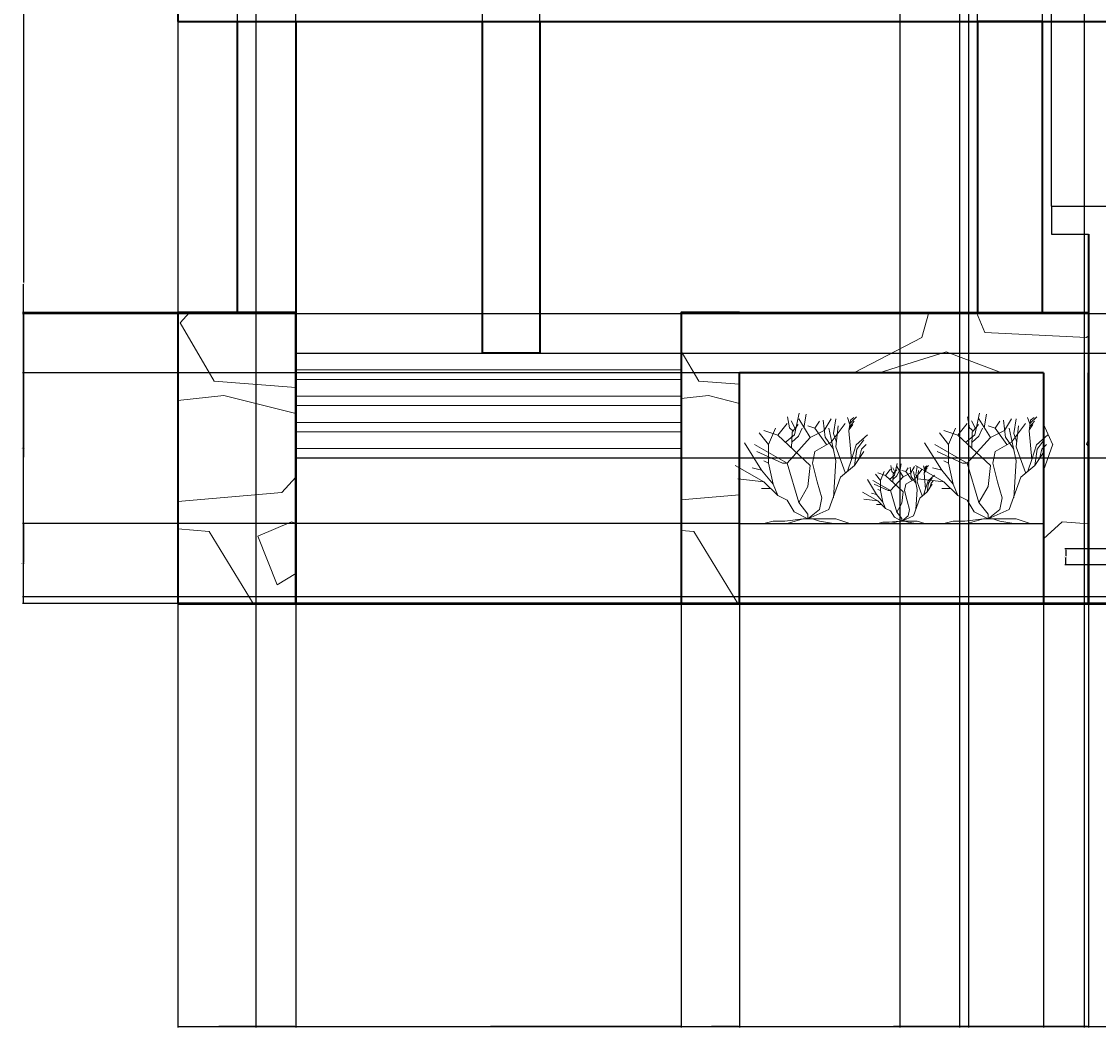
# Model space of a CAD drawing. Units: inches. Extents: x -8 to 554, y -200 to 499.
# Tile 1 of 12: x -8 to 214, y -200 to 7. Entities that reach past the tile are written whole.
import ezdxf

# ---------------------------------------------------------------- set-up
doc = ezdxf.new("R2010")
doc.units = ezdxf.units.IN
doc.header["$MEASUREMENT"] = 0
for name, color, linetype, lineweight in [('A-ANNO-DIMS', 2, 'Continuous', 18), ('A-COLS', 1, 'Continuous', 35), ('A-DOOR-GATE', 3, 'Continuous', 25), ('A-FLOR', 7, 'Continuous', 35), ('A-WALL', 7, 'Continuous', 35), ('A-WALL-PATT', 252, 'Continuous', 13), ('A-WALL-PRPT', 7, 'Continuous', 25), ('A-WALL-SCRN', 8, 'Continuous', 18), ('C-TOPO', 7, 'Continuous', 50), ('L-PLNT-TREE', 94, 'Continuous', 13)]:
    doc.layers.add(name, color=color, linetype=linetype, lineweight=lineweight)
doc.styles.get("Standard").update_dxf_attribs({"font": 'arial.ttf'})
doc.dimstyles.get("Standard").update_dxf_attribs({"dimtxt": 0.18, "dimasz": 0.18, "dimexe": 0.18, "dimexo": 0.0625, "dimgap": 0.09, "dimtad": 0, "dimtih": 1, "dimtoh": 1, "dimdec": 4, "dimzin": 0, "dimdsep": 46, "dimtxsty": 'Standard', "dimcen": 0.09, "dimadec": 0, "dimazin": 0, "dimtfac": 1, "dimtdec": 4, "dimtofl": 0, "dimtmove": 0, "dimatfit": 3, "dimfxl": 1, "dimtolj": 1, "dimtzin": 0, "dimarcsym": 0})

# ---------------------------------------------------------------- blocks, each defined once
blk = doc.blocks.new('*U2')
for p, q in [((-11.433, 18.289), (-10.457, 22.749)), ((-9.48, 19.775), (-8.992, 22.592)), ((-14.88, 18.24), (-12.96, 20.64)), ((-12.471, 19.775), (-12.898, 22.044)), ((-11.28, 19.619), (-12.104, 21.184)), ((-11.921, 18.836), (-10.64, 20.401)), ((-8.16, 17.76), (-10.56, 21.6)), ((-7.2, 19.68), (-8.64, 20.16)), ((-7.2, 19.68), (-6.24, 21.12)), ((-5.086, 17.741), (-5.513, 21.34)), ((-5.28, 19.2), (-3.84, 21.6)), ((-3.84, 16.8), (-0.96, 20.64)), ((-3.377, 18.602), (-2.888, 21.575)), ((-2.88, 15.84), (-2.4, 20.16)), ((-0.508, 21.888), (-0.081, 20.558)), ((-0.203, 19.149), (0.102, 21.34)), ((-0.142, 19.384), (0.59, 20.401)), ((-0.02, 20.01), (0.896, 21.105)), ((0.041, 20.714), (1.384, 22.044)), ((0.102, 21.34), (0.835, 21.888)), ((-16.8, 16.32), (-18.72, 18.72)), ((-14.88, 18.24), (-17.76, 19.2)), ((-16.8, 16.32), (-15.36, 19.68)), ((-8.16, 12), (-14.88, 18.24)), ((-13.325, 16.724), (-11.433, 18.289)), ((-11.677, 19.071), (-12.471, 19.775)), ((-12.043, 15.628), (-11.921, 18.836)), ((-11.982, 16.802), (-10.579, 18.054)), ((-10.579, 18.054), (-9.846, 19.697)), ((-8.16, 17.76), (-5.28, 19.2)), ((-4.8, 16.32), (-7.2, 19.68)), ((-3.377, 15.315), (-5.086, 17.819)), ((-2.88, 12.96), (-4.32, 19.68)), ((-2.766, 16.802), (-3.377, 18.602)), ((0.346, 13.203), (-0.203, 19.149)), ((1.323, 16.254), (3.642, 18.289)), ((-18.24, 11.04), (-21.755, 16.655)), ((-12.96, 12.48), (-19.68, 16.32)), ((-16.8, 12.48), (-16.8, 16.32)), ((-12.96, 12.48), (-8.16, 17.76)), ((-7.2, 14.88), (-3.84, 16.8)), ((-0.96, 10.56), (-2.88, 15.84)), ((0.346, 13.203), (1.323, 16.254)), ((1.44, 15.36), (2.88, 17.28)), ((2.4, 15.36), (3.36, 16.32)), ((-13.92, 12.48), (-19.2, 14.88)), ((-7.68, 12.48), (-7.2, 14.88)), ((0.96, 12), (1.44, 15.36)), ((0.96, 12), (2.88, 14.88)), ((1.92, 13.44), (2.4, 15.36)), ((-17.76, 8.64), (-23.663, 11.961)), ((-18.24, 11.04), (-20.16, 11.52)), ((-16.8, 12.48), (-17.76, 12.96)), ((-15.84, 8.16), (-16.8, 12.48)), ((-12.96, 12.48), (-13.92, 12.48)), ((-10.56, 4.32), (-12.96, 12.48)), ((-8.64, 7.68), (-8.16, 12)), ((-6.72, 8.64), (-7.68, 12.48)), ((-3.36, 5.28), (-2.88, 12.96)), ((-1.92, 9.6), (0.96, 12)), ((-0.48, 10.8), (0.346, 13.203)), ((-17.76, 8.64), (-23.128, 9.222)), ((-15.84, 8.16), (-18.24, 11.04)), ((-4.32, 2.88), (-1.92, 9.6)), ((-16.32, 7.2), (-18.24, 7.2)), ((-14.88, 5.76), (-17.76, 8.64)), ((-14.88, 5.76), (-15.84, 8.16)), ((-10.56, 4.32), (-8.64, 7.68)), ((-5.76, 5.28), (-6.72, 8.64)), ((-12.96, 4.8), (-14.88, 5.76)), ((-11.52, 2.4), (-12.96, 4.8)), ((-6.24, 2.88), (-5.76, 5.28)), ((-8.64, 0.96), (-11.52, 2.4)), ((-8.64, 1.92), (-10.56, 4.32)), ((-8.64, 0.96), (-4.32, 2.88)), ((-8.64, 0.96), (-6.24, 2.88)), ((-15.84, 0.48), (-17.76, 0)), ((-13.44, 0.48), (-15.84, 0.48)), ((-9.6, 0.96), (-13.44, 0.48)), ((-9.6, 0.96), (-12.96, 0)), ((-9.6, 0.96), (-7.68, 0.96)), ((-8.64, 0.96), (-8.64, 1.92)), ((-8.64, 0.96), (-2.88, 0.96)), ((-7.68, 0.96), (-6.24, 0.48)), ((-6.24, 0.48), (-3.36, 0)), ((-2.88, 0.96), (0, 0))]:
    blk.add_line(p, q)
blk = doc.blocks.new('GATE-PIER-ELEV')
blk.add_lwpolyline([(0, 76.14), (0, 0), (11.66, 0), (11.66, 76.14)])
blk = doc.blocks.new('*D15')
at = {"layer": 'A-ANNO-DIMS', "color": 0, "lineweight": -2, "transparency": 16777216}
for p, q in [((228.57, -101.26), (207.36, -101.26)), ((207.54, -101.44), (207.54, -102.71)), ((207.54, -104.35), (207.54, -103.08)), ((228.57, -104.53), (207.36, -104.53))]:
    blk.add_line(p, q, dxfattribs=at)
at = {"layer": 'A-ANNO-DIMS', "color": 0, "transparency": 16777216}
for points in [[(207.51, -101.44), (207.57, -101.44), (207.54, -101.26)], [(207.51, -104.35), (207.57, -104.35), (207.54, -104.53)]]:
    blk.add_solid(points, dxfattribs=at)
at = {"layer": 'Defpoints', "color": 0, "transparency": 16777216}
for p in [(207.54, -101.26), (228.63, -101.26), (228.63, -104.53)]:
    blk.add_point(p, dxfattribs=at)
at = {"layer": 'A-ANNO-DIMS', "color": 0, "transparency": 16777216, "insert": (207.54, -102.9), "char_height": 0.18, "attachment_point": 5}
blk.add_mtext('\\A1;3 TYP.', dxfattribs=at)
blk = doc.blocks.new('*D31')
at = {"layer": 'A-ANNO-DIMS', "color": 0, "lineweight": -2, "transparency": 16777216}
for p, q in [((24.34, 127.42), (24.34, -199.97)), ((453.32, -30.73), (453.32, -199.97)), ((24.52, -199.79), (238.54, -199.79)), ((453.14, -199.79), (239.12, -199.79))]:
    blk.add_line(p, q, dxfattribs=at)
at = {"layer": 'A-ANNO-DIMS', "color": 0, "transparency": 16777216}
for points in [[(24.52, -199.76), (24.52, -199.82), (24.34, -199.79)], [(453.14, -199.76), (453.14, -199.82), (453.32, -199.79)]]:
    blk.add_solid(points, dxfattribs=at)
at = {"layer": 'Defpoints', "color": 0, "transparency": 16777216}
for p in [(24.34, 127.48), (453.32, -30.67), (453.32, -199.79)]:
    blk.add_point(p, dxfattribs=at)
at = {"layer": 'A-ANNO-DIMS', "color": 0, "transparency": 16777216, "insert": (238.83, -199.79), "char_height": 0.18, "attachment_point": 5}
blk.add_mtext('\\A1;429', dxfattribs=at)
blk = doc.blocks.new('*D32')
at = {"layer": 'A-ANNO-DIMS', "color": 0, "lineweight": -2, "transparency": 16777216}
for p, q in [((24.34, 223.42), (24.34, -199.97)), ((444.34, 223.42), (444.34, -199.97)), ((24.52, -199.79), (234.05, -199.79)), ((444.16, -199.79), (234.63, -199.79))]:
    blk.add_line(p, q, dxfattribs=at)
at = {"layer": 'A-ANNO-DIMS', "color": 0, "transparency": 16777216}
for points in [[(24.52, -199.76), (24.52, -199.82), (24.34, -199.79)], [(444.16, -199.76), (444.16, -199.82), (444.34, -199.79)]]:
    blk.add_solid(points, dxfattribs=at)
at = {"layer": 'Defpoints', "color": 0, "transparency": 16777216}
for p in [(24.34, 223.48), (444.34, 223.48), (444.34, -199.79)]:
    blk.add_point(p, dxfattribs=at)
at = {"layer": 'A-ANNO-DIMS', "color": 0, "transparency": 16777216, "insert": (234.34, -199.79), "char_height": 0.18, "attachment_point": 5}
blk.add_mtext('\\A1;420', dxfattribs=at)
blk = doc.blocks.new('*D33')
at = {"layer": 'A-ANNO-DIMS', "color": 0, "lineweight": -2, "transparency": 16777216}
for p, q in [((36.28, 19.48), (-7.69, 19.48)), ((-7.51, 19.3), (-7.51, -46.34)), ((-7.51, -112.34), (-7.51, -46.7)), ((24.28, -112.52), (-7.69, -112.52))]:
    blk.add_line(p, q, dxfattribs=at)
at = {"layer": 'A-ANNO-DIMS', "color": 0, "transparency": 16777216}
for points in [[(-7.54, 19.3), (-7.48, 19.3), (-7.51, 19.48)], [(-7.54, -112.34), (-7.48, -112.34), (-7.51, -112.52)]]:
    blk.add_solid(points, dxfattribs=at)
at = {"layer": 'Defpoints', "color": 0, "transparency": 16777216}
for p in [(-7.51, 19.48), (36.34, 19.48), (24.34, -112.52)]:
    blk.add_point(p, dxfattribs=at)
at = {"layer": 'A-ANNO-DIMS', "color": 0, "transparency": 16777216, "insert": (-7.51, -46.52), "char_height": 0.18, "attachment_point": 5}
blk.add_mtext('\\A1;132', dxfattribs=at)
blk = doc.blocks.new('*D41')
at = {"layer": 'A-ANNO-DIMS', "color": 0, "lineweight": -2, "transparency": 16777216}
for p, q in [((24.34, 235.42), (24.34, -199.97)), ((40.45, 235.42), (40.45, -199.97)), ((24.52, -199.79), (31.94, -199.79)), ((40.27, -199.79), (32.85, -199.79))]:
    blk.add_line(p, q, dxfattribs=at)
at = {"layer": 'A-ANNO-DIMS', "color": 0, "transparency": 16777216}
for points in [[(24.52, -199.76), (24.52, -199.82), (24.34, -199.79)], [(40.27, -199.76), (40.27, -199.82), (40.45, -199.79)]]:
    blk.add_solid(points, dxfattribs=at)
at = {"layer": 'Defpoints', "color": 0, "transparency": 16777216}
for p in [(24.34, 235.48), (40.45, 235.48), (40.45, -199.79)]:
    blk.add_point(p, dxfattribs=at)
at = {"layer": 'A-ANNO-DIMS', "color": 0, "transparency": 16777216, "insert": (32.4, -199.79), "char_height": 0.18, "attachment_point": 5}
blk.add_mtext('\\A1;16.113', dxfattribs=at)
blk = doc.blocks.new('*D48')
at = {"layer": 'A-ANNO-DIMS', "color": 0, "lineweight": -2, "transparency": 16777216}
for p, q in [((24.34, -112.58), (24.34, -199.97)), ((48.69, -112.58), (48.69, -199.97)), ((24.52, -199.79), (36.05, -199.79)), ((48.51, -199.79), (36.98, -199.79))]:
    blk.add_line(p, q, dxfattribs=at)
at = {"layer": 'A-ANNO-DIMS', "color": 0, "transparency": 16777216}
for points in [[(24.52, -199.76), (24.52, -199.82), (24.34, -199.79)], [(48.51, -199.76), (48.51, -199.82), (48.69, -199.79)]]:
    blk.add_solid(points, dxfattribs=at)
at = {"layer": 'Defpoints', "color": 0, "transparency": 16777216}
for p in [(24.34, -112.52), (48.69, -112.52), (48.69, -199.79)]:
    blk.add_point(p, dxfattribs=at)
at = {"layer": 'A-ANNO-DIMS', "color": 0, "transparency": 16777216, "insert": (36.52, -199.79), "char_height": 0.18, "attachment_point": 5}
blk.add_mtext('\\A1;24.346', dxfattribs=at)
blk = doc.blocks.new('*D49')
at = {"layer": 'A-ANNO-DIMS', "color": 0, "lineweight": -2, "transparency": 16777216}
for p, q in [((48.69, -112.58), (48.69, -199.97)), ((128.23, -112.58), (128.23, -199.97)), ((48.87, -199.79), (88.07, -199.79)), ((128.05, -199.79), (88.85, -199.79))]:
    blk.add_line(p, q, dxfattribs=at)
at = {"layer": 'A-ANNO-DIMS', "color": 0, "transparency": 16777216}
for points in [[(48.87, -199.76), (48.87, -199.82), (48.69, -199.79)], [(128.05, -199.76), (128.05, -199.82), (128.23, -199.79)]]:
    blk.add_solid(points, dxfattribs=at)
at = {"layer": 'Defpoints', "color": 0, "transparency": 16777216}
for p in [(48.69, -112.52), (128.23, -112.52), (128.23, -199.79)]:
    blk.add_point(p, dxfattribs=at)
at = {"layer": 'A-ANNO-DIMS', "color": 0, "transparency": 16777216, "insert": (88.46, -199.79), "char_height": 0.18, "attachment_point": 5}
blk.add_mtext('\\A1;79.54', dxfattribs=at)
blk = doc.blocks.new('*D50')
at = {"layer": 'A-ANNO-DIMS', "color": 0, "lineweight": -2, "transparency": 16777216}
for p, q in [((128.23, -112.58), (128.23, -199.97)), ((140.23, -112.58), (140.23, -199.97)), ((128.41, -199.79), (134.02, -199.79)), ((140.05, -199.79), (134.44, -199.79))]:
    blk.add_line(p, q, dxfattribs=at)
at = {"layer": 'A-ANNO-DIMS', "color": 0, "transparency": 16777216}
for points in [[(128.41, -199.76), (128.41, -199.82), (128.23, -199.79)], [(140.05, -199.76), (140.05, -199.82), (140.23, -199.79)]]:
    blk.add_solid(points, dxfattribs=at)
at = {"layer": 'Defpoints', "color": 0, "transparency": 16777216}
for p in [(128.23, -112.52), (140.23, -112.52), (140.23, -199.79)]:
    blk.add_point(p, dxfattribs=at)
at = {"layer": 'A-ANNO-DIMS', "color": 0, "transparency": 16777216, "insert": (134.23, -199.79), "char_height": 0.18, "attachment_point": 5}
blk.add_mtext('\\A1;12', dxfattribs=at)
blk = doc.blocks.new('*D51')
at = {"layer": 'A-ANNO-DIMS', "color": 0, "lineweight": -2, "transparency": 16777216}
for p, q in [((140.23, -112.58), (140.23, -199.97)), ((202.92, -112.58), (202.92, -199.97)), ((140.41, -199.79), (171.18, -199.79)), ((202.74, -199.79), (171.97, -199.79))]:
    blk.add_line(p, q, dxfattribs=at)
at = {"layer": 'A-ANNO-DIMS', "color": 0, "transparency": 16777216}
for points in [[(140.41, -199.76), (140.41, -199.82), (140.23, -199.79)], [(202.74, -199.76), (202.74, -199.82), (202.92, -199.79)]]:
    blk.add_solid(points, dxfattribs=at)
at = {"layer": 'Defpoints', "color": 0, "transparency": 16777216}
for p in [(140.23, -112.52), (202.92, -112.52), (202.92, -199.79)]:
    blk.add_point(p, dxfattribs=at)
at = {"layer": 'A-ANNO-DIMS', "color": 0, "transparency": 16777216, "insert": (171.57, -199.79), "char_height": 0.18, "attachment_point": 5}
blk.add_mtext('\\A1;62.69', dxfattribs=at)
blk = doc.blocks.new('*D52')
at = {"layer": 'A-ANNO-DIMS', "color": 0, "lineweight": -2, "transparency": 16777216}
for p, q in [((202.92, -112.58), (202.92, -199.97)), ((212.23, -112.58), (212.23, -199.97)), ((203.1, -199.79), (207.18, -199.79)), ((212.05, -199.79), (207.97, -199.79))]:
    blk.add_line(p, q, dxfattribs=at)
at = {"layer": 'A-ANNO-DIMS', "color": 0, "transparency": 16777216}
for points in [[(203.1, -199.76), (203.1, -199.82), (202.92, -199.79)], [(212.05, -199.76), (212.05, -199.82), (212.23, -199.79)]]:
    blk.add_solid(points, dxfattribs=at)
at = {"layer": 'Defpoints', "color": 0, "transparency": 16777216}
for p in [(202.92, -112.52), (212.23, -112.52), (212.23, -199.79)]:
    blk.add_point(p, dxfattribs=at)
at = {"layer": 'A-ANNO-DIMS', "color": 0, "transparency": 16777216, "insert": (207.57, -199.79), "char_height": 0.18, "attachment_point": 5}
blk.add_mtext('\\A1;9.307', dxfattribs=at)
blk = doc.blocks.new('*D54')
at = {"layer": 'A-ANNO-DIMS', "color": 0, "lineweight": -2, "transparency": 16777216}
for p, q in [((24.28, -52.52), (-7.69, -52.52)), ((-7.51, -52.7), (-7.51, -82.34)), ((-7.51, -112.34), (-7.51, -82.7)), ((24.28, -112.52), (-7.69, -112.52))]:
    blk.add_line(p, q, dxfattribs=at)
at = {"layer": 'A-ANNO-DIMS', "color": 0, "transparency": 16777216}
for points in [[(-7.54, -52.7), (-7.48, -52.7), (-7.51, -52.52)], [(-7.54, -112.34), (-7.48, -112.34), (-7.51, -112.52)]]:
    blk.add_solid(points, dxfattribs=at)
at = {"layer": 'Defpoints', "color": 0, "transparency": 16777216}
for p in [(-7.51, -52.52), (24.34, -52.52), (24.34, -112.52)]:
    blk.add_point(p, dxfattribs=at)
at = {"layer": 'A-ANNO-DIMS', "color": 0, "transparency": 16777216, "insert": (-7.51, -82.52), "char_height": 0.18, "attachment_point": 5}
blk.add_mtext('\\A1;60', dxfattribs=at)
blk = doc.blocks.new('*D55')
at = {"layer": 'A-ANNO-DIMS', "color": 0, "lineweight": -2, "transparency": 16777216}
for p, q in [((204.61, -30.61), (204.61, 498.99)), ((204.79, 498.81), (328.57, 498.81)), ((453.14, 498.81), (329.36, 498.81)), ((453.32, -30.61), (453.32, 498.99))]:
    blk.add_line(p, q, dxfattribs=at)
at = {"layer": 'A-ANNO-DIMS', "color": 0, "transparency": 16777216}
for points in [[(204.79, 498.84), (204.79, 498.78), (204.61, 498.81)], [(453.14, 498.84), (453.14, 498.78), (453.32, 498.81)]]:
    blk.add_solid(points, dxfattribs=at)
at = {"layer": 'Defpoints', "color": 0, "transparency": 16777216}
for p in [(453.32, 498.81), (204.61, -30.67), (453.32, -30.67)]:
    blk.add_point(p, dxfattribs=at)
at = {"layer": 'A-ANNO-DIMS', "color": 0, "transparency": 16777216, "insert": (328.96, 498.81), "char_height": 0.18, "attachment_point": 5}
blk.add_mtext('\\A1;248.7', dxfattribs=at)
blk = doc.blocks.new('*D57')
at = {"layer": 'A-ANNO-DIMS', "color": 0, "lineweight": -2, "transparency": 16777216}
for p, q in [((36.69, -52.46), (36.69, 498.99)), ((36.87, 498.81), (42.48, 498.81)), ((48.51, 498.81), (42.9, 498.81)), ((48.69, -52.46), (48.69, 498.99))]:
    blk.add_line(p, q, dxfattribs=at)
at = {"layer": 'A-ANNO-DIMS', "color": 0, "transparency": 16777216}
for points in [[(36.87, 498.84), (36.87, 498.78), (36.69, 498.81)], [(48.51, 498.84), (48.51, 498.78), (48.69, 498.81)]]:
    blk.add_solid(points, dxfattribs=at)
at = {"layer": 'Defpoints', "color": 0, "transparency": 16777216}
for p in [(48.69, 498.81), (36.69, -52.52), (48.69, -52.52)]:
    blk.add_point(p, dxfattribs=at)
at = {"layer": 'A-ANNO-DIMS', "color": 0, "transparency": 16777216, "insert": (42.69, 498.81), "char_height": 0.18, "attachment_point": 5}
blk.add_mtext('\\A1;12', dxfattribs=at)
blk = doc.blocks.new('*D59')
at = {"layer": 'A-ANNO-DIMS', "color": 0, "lineweight": -2, "transparency": 16777216}
for p, q in [((87.21, -60.84), (87.21, 498.99)), ((87.39, 498.81), (92.67, 498.81)), ((98.86, 498.81), (93.58, 498.81)), ((99.04, -60.84), (99.04, 498.99))]:
    blk.add_line(p, q, dxfattribs=at)
at = {"layer": 'A-ANNO-DIMS', "color": 0, "transparency": 16777216}
for points in [[(87.39, 498.84), (87.39, 498.78), (87.21, 498.81)], [(98.86, 498.84), (98.86, 498.78), (99.04, 498.81)]]:
    blk.add_solid(points, dxfattribs=at)
at = {"layer": 'Defpoints', "color": 0, "transparency": 16777216}
for p in [(99.04, 498.81), (87.21, -60.9), (99.04, -60.9)]:
    blk.add_point(p, dxfattribs=at)
at = {"layer": 'A-ANNO-DIMS', "color": 0, "transparency": 16777216, "insert": (93.12, 498.81), "char_height": 0.18, "attachment_point": 5}
blk.add_mtext('\\A1;11.827', dxfattribs=at)
blk = doc.blocks.new('*D61')
at = {"layer": 'A-ANNO-DIMS', "color": 0, "lineweight": -2, "transparency": 16777216}
for p, q in [((189.3, -52.46), (189.3, 498.99)), ((189.48, 498.81), (195.57, 498.81)), ((202.57, 498.81), (196.48, 498.81)), ((202.75, -52.46), (202.75, 498.99))]:
    blk.add_line(p, q, dxfattribs=at)
at = {"layer": 'A-ANNO-DIMS', "color": 0, "transparency": 16777216}
for points in [[(189.48, 498.84), (189.48, 498.78), (189.3, 498.81)], [(202.57, 498.84), (202.57, 498.78), (202.75, 498.81)]]:
    blk.add_solid(points, dxfattribs=at)
at = {"layer": 'Defpoints', "color": 0, "transparency": 16777216}
for p in [(202.75, 498.81), (189.3, -52.52), (202.75, -52.52)]:
    blk.add_point(p, dxfattribs=at)
at = {"layer": 'A-ANNO-DIMS', "color": 0, "transparency": 16777216, "insert": (196.03, 498.81), "char_height": 0.18, "attachment_point": 5}
blk.add_mtext('\\A1;13.446', dxfattribs=at)
blk = doc.blocks.new('*D66')
at = {"layer": 'A-ANNO-DIMS', "color": 0, "lineweight": -2, "transparency": 16777216}
for p, q in [((225.57, -52.82), (-7.69, -52.82)), ((-7.51, -53), (-7.51, -81.79)), ((-7.51, -110.95), (-7.51, -82.16)), ((225.57, -111.13), (-7.69, -111.13))]:
    blk.add_line(p, q, dxfattribs=at)
at = {"layer": 'A-ANNO-DIMS', "color": 0, "transparency": 16777216}
for points in [[(-7.54, -53), (-7.48, -53), (-7.51, -52.82)], [(-7.54, -110.95), (-7.48, -110.95), (-7.51, -111.13)]]:
    blk.add_solid(points, dxfattribs=at)
at = {"layer": 'Defpoints', "color": 0, "transparency": 16777216}
for p in [(225.63, -52.82), (-7.51, -111.13), (225.63, -111.13)]:
    blk.add_point(p, dxfattribs=at)
at = {"layer": 'A-ANNO-DIMS', "color": 0, "transparency": 16777216, "insert": (-7.51, -81.98), "char_height": 0.18, "attachment_point": 5}
blk.add_mtext('\\A1;58.3', dxfattribs=at)
blk = doc.blocks.new('*D74')
at = {"layer": 'A-ANNO-DIMS', "color": 0, "lineweight": -2, "transparency": 16777216}
for p, q in [((140.17, -96.01), (-7.69, -96.01)), ((-7.51, -96.19), (-7.51, -104.08)), ((-7.51, -112.34), (-7.51, -104.45)), ((140.17, -112.52), (-7.69, -112.52))]:
    blk.add_line(p, q, dxfattribs=at)
at = {"layer": 'A-ANNO-DIMS', "color": 0, "transparency": 16777216}
for points in [[(-7.54, -96.19), (-7.48, -96.19), (-7.51, -96.01)], [(-7.54, -112.34), (-7.48, -112.34), (-7.51, -112.52)]]:
    blk.add_solid(points, dxfattribs=at)
at = {"layer": 'Defpoints', "color": 0, "transparency": 16777216}
for p in [(-7.51, -96.01), (140.23, -96.01), (140.23, -112.52)]:
    blk.add_point(p, dxfattribs=at)
at = {"layer": 'A-ANNO-DIMS', "color": 0, "transparency": 16777216, "insert": (-7.51, -104.27), "char_height": 0.18, "attachment_point": 5}
blk.add_mtext('\\A1;16.507', dxfattribs=at)
blk = doc.blocks.new('*D75')
at = {"layer": 'A-ANNO-DIMS', "color": 0, "lineweight": -2, "transparency": 16777216}
for p, q in [((140.17, -64.97), (-7.69, -64.97)), ((-7.51, -65.15), (-7.51, -80.31)), ((-7.51, -95.83), (-7.51, -80.67)), ((140.17, -96.01), (-7.69, -96.01))]:
    blk.add_line(p, q, dxfattribs=at)
at = {"layer": 'A-ANNO-DIMS', "color": 0, "transparency": 16777216}
for points in [[(-7.54, -65.15), (-7.48, -65.15), (-7.51, -64.97)], [(-7.54, -95.83), (-7.48, -95.83), (-7.51, -96.01)]]:
    blk.add_solid(points, dxfattribs=at)
at = {"layer": 'Defpoints', "color": 0, "transparency": 16777216}
for p in [(-7.51, -64.97), (140.23, -64.97), (140.23, -96.01)]:
    blk.add_point(p, dxfattribs=at)
at = {"layer": 'A-ANNO-DIMS', "color": 0, "transparency": 16777216, "insert": (-7.51, -80.49), "char_height": 0.18, "attachment_point": 5}
blk.add_mtext('\\A1;31.045', dxfattribs=at)
blk = doc.blocks.new('*D76')
at = {"layer": 'A-ANNO-DIMS', "color": 0, "lineweight": -2, "transparency": 16777216}
for p, q in [((48.75, -82.52), (554.26, -82.52)), ((554.08, -82.7), (554.08, -97.34)), ((554.08, -112.34), (554.08, -97.7)), ((48.75, -112.52), (554.26, -112.52))]:
    blk.add_line(p, q, dxfattribs=at)
at = {"layer": 'A-ANNO-DIMS', "color": 0, "transparency": 16777216}
for points in [[(554.05, -82.7), (554.11, -82.7), (554.08, -82.52)], [(554.05, -112.34), (554.11, -112.34), (554.08, -112.52)]]:
    blk.add_solid(points, dxfattribs=at)
at = {"layer": 'Defpoints', "color": 0, "transparency": 16777216}
for p in [(48.69, -82.52), (554.08, -82.52), (48.69, -112.52)]:
    blk.add_point(p, dxfattribs=at)
at = {"layer": 'A-ANNO-DIMS', "color": 0, "transparency": 16777216, "insert": (554.08, -97.52), "char_height": 0.18, "attachment_point": 5}
blk.add_mtext('\\A1;30', dxfattribs=at)
blk = doc.blocks.new('*D77')
at = {"layer": 'A-ANNO-DIMS', "color": 0, "lineweight": -2, "transparency": 16777216}
for p, q in [((48.75, -60.9), (554.26, -60.9)), ((554.08, -61.08), (554.08, -71.53)), ((554.08, -82.34), (554.08, -71.89)), ((48.75, -82.52), (554.26, -82.52))]:
    blk.add_line(p, q, dxfattribs=at)
at = {"layer": 'A-ANNO-DIMS', "color": 0, "transparency": 16777216}
for points in [[(554.05, -61.08), (554.11, -61.08), (554.08, -60.9)], [(554.05, -82.34), (554.11, -82.34), (554.08, -82.52)]]:
    blk.add_solid(points, dxfattribs=at)
at = {"layer": 'Defpoints', "color": 0, "transparency": 16777216}
for p in [(48.69, -60.9), (554.08, -60.9), (48.69, -82.52)]:
    blk.add_point(p, dxfattribs=at)
at = {"layer": 'A-ANNO-DIMS', "color": 0, "transparency": 16777216, "insert": (554.08, -71.71), "char_height": 0.18, "attachment_point": 5}
blk.add_mtext('\\A1;21.615', dxfattribs=at)
blk = doc.blocks.new('*D80')
at = {"layer": 'A-ANNO-DIMS', "color": 0, "lineweight": -2, "transparency": 16777216}
for p, q in [((173.34, 314.42), (173.34, -199.97)), ((211.34, 314.42), (211.34, -199.97)), ((173.52, -199.79), (192.12, -199.79)), ((211.16, -199.79), (192.56, -199.79))]:
    blk.add_line(p, q, dxfattribs=at)
at = {"layer": 'A-ANNO-DIMS', "color": 0, "transparency": 16777216}
for points in [[(173.52, -199.76), (173.52, -199.82), (173.34, -199.79)], [(211.16, -199.76), (211.16, -199.82), (211.34, -199.79)]]:
    blk.add_solid(points, dxfattribs=at)
at = {"layer": 'Defpoints', "color": 0, "transparency": 16777216}
for p in [(173.34, 314.48), (211.34, 314.48), (211.34, -199.79)]:
    blk.add_point(p, dxfattribs=at)
at = {"layer": 'A-ANNO-DIMS', "color": 0, "transparency": 16777216, "insert": (192.34, -199.79), "char_height": 0.18, "attachment_point": 5}
blk.add_mtext('\\A1;38', dxfattribs=at)
blk = doc.blocks.new('*D81')
at = {"layer": 'A-ANNO-DIMS', "color": 0, "lineweight": -2, "transparency": 16777216}
for p, q in [((173.34, 235.42), (173.34, -199.97)), ((185.64, 235.42), (185.64, -199.97)), ((173.52, -199.79), (179.04, -199.79)), ((185.46, -199.79), (179.95, -199.79))]:
    blk.add_line(p, q, dxfattribs=at)
at = {"layer": 'A-ANNO-DIMS', "color": 0, "transparency": 16777216}
for points in [[(173.52, -199.76), (173.52, -199.82), (173.34, -199.79)], [(185.46, -199.76), (185.46, -199.82), (185.64, -199.79)]]:
    blk.add_solid(points, dxfattribs=at)
at = {"layer": 'Defpoints', "color": 0, "transparency": 16777216}
for p in [(173.34, 235.48), (185.64, 235.48), (185.64, -199.79)]:
    blk.add_point(p, dxfattribs=at)
at = {"layer": 'A-ANNO-DIMS', "color": 0, "transparency": 16777216, "insert": (179.49, -199.79), "char_height": 0.18, "attachment_point": 5}
blk.add_mtext('\\A1;12.302', dxfattribs=at)
blk = doc.blocks.new('*D82')
at = {"layer": 'A-ANNO-DIMS', "color": 0, "lineweight": -2, "transparency": 16777216}
for p, q in [((185.64, 235.42), (185.64, -199.97)), ((187.48, 235.42), (187.48, -199.97)), ((185.82, -199.79), (186.18, -199.79)), ((187.3, -199.79), (186.95, -199.79))]:
    blk.add_line(p, q, dxfattribs=at)
at = {"layer": 'A-ANNO-DIMS', "color": 0, "transparency": 16777216}
for points in [[(185.82, -199.76), (185.82, -199.82), (185.64, -199.79)], [(187.3, -199.76), (187.3, -199.82), (187.48, -199.79)]]:
    blk.add_solid(points, dxfattribs=at)
at = {"layer": 'Defpoints', "color": 0, "transparency": 16777216}
for p in [(185.64, 235.48), (187.48, 235.48), (187.48, -199.79)]:
    blk.add_point(p, dxfattribs=at)
at = {"layer": 'A-ANNO-DIMS', "color": 0, "transparency": 16777216, "insert": (186.56, -199.79), "char_height": 0.18, "attachment_point": 5}
blk.add_mtext('\\A1;1.837', dxfattribs=at)

msp = doc.modelspace()

# ---------------------------------------------------------------- hatches: boundary and pattern name
at = {"layer": 'A-WALL-PATT'}
h = msp.add_hatch(dxfattribs=at)
h.set_pattern_fill('GRAVEL', color=256, scale=100)
h.set_pattern_definition([(228.0128, (-45.809, 19.688), (-800, -900), [13.4536, -1331.909]), (184.9697, (-54.8087, 9.688), (1200, 100), [23.0868, -2285.5925]), (132.5104, (-77.809, 7.688), (1000, -1100), [16.279, -1611.6033]), (267.2737, (-116.8087, -17.312), (100, 2000), [21.0238, -2081.3558]), (292.83365, (-117.8087, -38.312), (-500, 1200), [20.6155, -2040.9373]), (357.2737, (-109.8087, -57.312), (-2000, 100), [21.0238, -2081.3558]), (37.69424, (-88.8087, -58.3118), (-1300, -1000), [27.803, -2752.4849]), (72.2553, (-66.8087, -41.312), (700, 2200), [26.2488, -2598.632]), (121.4296, (-58.8087, -16.312), (-800, 1300), [21.095, -2088.4073]), (175.2364, (-69.809, 1.688), (1100, -100), [24.083, -1180.076]), (222.39744, (-93.8087, 3.6882), (-1200, -1100), [31.1448, -3083.3375]), (138.814, (-17.809, -18.312), (-700, 600), [10.63, -1052.3845]), (171.4692, (-25.8087, -11.312), (1300, -200), [20.2237, -2002.151]), (225, (-45.81, -8.31), (-1e-14, -100), [14.142, -127.279]), (203.1986, (-52.809, 3.688), (500, 200), [7.616, -753.9615]), (291.8014, (-59.809, 0.688), (-100, 300), [10.77, -527.746]), (30.9638, (-55.809, -9.312), (300, 200), [17.493, -565.602]), (161.565, (-40.81, -0.312), (200, -100), [12.649, -303.579]), (16.3895, (-117.8087, 0.688), (1000, 300), [17.72, -1754.2845]), (70.3462, (-100.809, 5.688), (-400, -1100), [14.866, -1471.741]), (293.1986, (-40.809, 19.688), (-200, 500), [15.2315, -746.346]), (343.6105, (-34.8087, 5.688), (-1000, 300), [17.72, -1754.2845]), (339.444, (-117.809, -61.312), (-500, 200), [17.088, -837.3124]), (294.7751, (-101.809, -67.312), (-500, 1100), [14.318, -1417.4643]), (66.8014, (-39.809, -80.312), (200, 500), [15.2315, -746.346]), (17.354, (-33.809, -66.312), (-1300, -400), [16.763, -1659.5424]), (69.444, (-88.809, -80.312), (-200, -500), [8.544, -845.8564]), (101.31, (-45.809, -80.312), (-100, 400), [5.099, -504.803]), (165.9638, (-46.809, -75.312), (300, -100), [20.6155, -391.695]), (186.009, (-66.8087, -70.312), (1000, 100), [19.105, -1891.3923]), (303.69, (-55.81, -18.312), (-100, 200), [14.422, -346.133]), (353.1572, (-47.8087, -30.312), (1700, -200), [25.1794, -2492.7563]), (60.9454, (-22.809, -33.312), (-400, -700), [10.2956, -1019.2674]), (90, (-17.81, -24.31), (-100, 100), [6, -94]), (120.2564, (-68.809, -67.312), (400, -700), [13.8924, -1375.352]), (48.0128, (-75.809, -55.312), (800, 900), [26.907, -1318.455]), (0, (-57.81, -35.31), (100, 100), [26, -74]), (325.3048, (-31.809, -35.312), (1000, -700), [15.8114, -1565.3274]), (254.0546, (-18.809, -44.312), (-100, -400), [14.56, -713.451]), (207.646, (-22.8087, -58.312), (-1900, -1000), [23.7065, -2346.9474]), (175.4261, (-43.8087, -69.312), (-1300, 100), [25.08, -2482.9073])])
h.paths.add_polyline_path([(48.6882, -52.5186), (24.3421, -52.5186), (24.3421, -112.5186), (48.6882, -112.5186)])
h.paths.add_polyline_path([(212.2282, -52.5186), (140.2282, -52.5186), (128.2282, -52.5186), (128.2282, -112.5186), (140.2282, -112.5186), (140.2282, -64.9665), (202.9211, -64.9665), (202.9211, -112.5186), (212.2282, -112.5186)])
h.paths.add_polyline_path([(312.3421, 49.7921), (216.3421, 49.7921), (216.3421, 19.4814), (312.3421, 19.4814)])
h.paths.add_polyline_path([(312.3421, 157.7921), (216.3421, 157.7921), (216.3421, 127.4814), (312.3421, 127.4814)])
h.paths.add_polyline_path([(312.3421, 265.7921), (216.3421, 265.7921), (216.3421, 235.4814), (312.3421, 235.4814)])
h.paths.add_polyline_path([(432.5174, 371.7921), (215.6778, 371.7921), (215.6778, 368.5162), (215.6778, 357.6367), (35.7874, 357.6367), (35.7874, 360.9127), (35.7874, 371.7921), (24.3421, 371.7921), (24.3421, 343.4814), (35.7874, 343.4814), (432.5174, 343.4814)])

# ---------------------------------------------------------------- linework, layer by layer
at = {"layer": 'A-COLS'}
msp.add_lwpolyline([(36.6882, -52.5186), (36.6882, 7.4814), (48.6882, 7.4814), (48.6882, -112.5186), (36.6882, -112.5186)], dxfattribs=at)
for points in [[(87.21, 7.4814), (99.037, 7.4814), (99.037, -60.9032), (87.21, -60.9032)], [(202.7513, 7.4814), (189.3049, 7.4814), (189.3049, -52.5186), (202.7513, -52.5186)]]:
    msp.add_lwpolyline(points, close=True, dxfattribs=at)
at = {"layer": 'A-DOOR-GATE'}
msp.add_lwpolyline([(446.0855, -36.3739), (453.3222, -36.3739), (453.3222, -30.6677), (204.6055, -30.6677), (204.6055, -36.3739), (212.2282, -36.3739)], dxfattribs=at)
at = {"layer": 'A-FLOR'}
msp.add_line((24.3421, 7.4814), (444.3421, 7.4814), dxfattribs=at)
at = {"layer": 'A-WALL'}
msp.add_line((24.3421, 127.4814), (24.3421, 7.4814), dxfattribs=at)
msp.add_lwpolyline([(24.3421, -112.5186), (48.6882, -112.5186), (48.6882, -52.5186), (24.3421, -52.5186)], close=True, dxfattribs=at)
for points in [[(140.2282, -52.5186), (128.2282, -52.5186), (128.2282, -112.5186), (140.2282, -112.5186), (140.2282, -64.9665)], [(140.2282, -52.5186), (212.2282, -52.5186), (212.2282, -64.9665)], [(202.9211, -64.9665), (140.2282, -64.9665)], [(202.9211, -64.9665), (202.9211, -112.5186), (212.2282, -112.5186), (212.2282, -64.9665)]]:
    msp.add_lwpolyline(points, dxfattribs=at)
at = {"layer": 'A-WALL-PRPT'}
msp.add_line((140.2282, -96.0119), (202.9211, -96.0119), dxfattribs=at)
at = {"layer": 'A-WALL-SCRN'}
for points in [[(48.6882, -64.3796), (128.2282, -64.3796), (128.2282, -60.9032), (48.6882, -60.9032)], [(48.6882, -69.7834), (128.2282, -69.7834), (128.2282, -66.3071), (48.6882, -66.3071)], [(48.6882, -75.1873), (128.2282, -75.1873), (128.2282, -71.7109), (48.6882, -71.7109)], [(48.6882, -80.5911), (128.2282, -80.5911), (128.2282, -77.1148), (48.6882, -77.1148)], [(48.6882, -82.5186), (128.2282, -82.5186), (128.2282, -112.5186), (48.6882, -112.5186)]]:
    msp.add_lwpolyline(points, close=True, dxfattribs=at)
at = {"layer": 'C-TOPO'}
msp.add_line((24.3421, -112.5186), (522.2333, -112.5186), dxfattribs=at)

# ---------------------------------------------------------------- block references
at = {"layer": 'A-COLS'}
msp.add_blockref('GATE-PIER-ELEV', (212.2282, -112.5186), dxfattribs=at)
at = {"layer": 'L-PLNT-TREE'}
for p in [(163.0004, -96.0542), (200.1797, -96.0542)]:
    msp.add_blockref('*U2', p, dxfattribs=at)
at = {"layer": 'L-PLNT-TREE', "xscale": 0.5440329233585479, "yscale": 0.5440329233585479, "zscale": 0.5440329233585479}
msp.add_blockref('*U2', (178.4459, -96.0542), dxfattribs=at)

# ---------------------------------------------------------------- dimensions: what is measured, and where the dimension line sits
at = {"layer": 'A-ANNO-DIMS'}
for base, p1, p2, override, picture, middle in [((48.6882, 498.8091), (36.6882, -52.5186), (48.6882, -52.5186), {"dimdec": 0, "dimlfac": 1, "dimrnd": 0, "dimzin": 0, "dimdsep": 46, "dimlunit": 2}, '*D57', (42.6882, 498.8091)), ((99.037, 498.8091), (87.21, -60.9032), (99.037, -60.9032), {"dimdec": 3, "dimlfac": 1, "dimrnd": 0, "dimzin": 0, "dimdsep": 46, "dimlunit": 2}, '*D59', (93.1235, 498.8091)), ((202.7513, 498.8091), (189.3049, -52.5186), (202.7513, -52.5186), {"dimdec": 3, "dimlfac": 1, "dimrnd": 0, "dimzin": 0, "dimdsep": 46, "dimlunit": 2}, '*D61', (196.0281, 498.8091)), ((453.3222, 498.8091), (204.6055, -30.6677), (453.3222, -30.6677), {"dimdec": 1, "dimlfac": 1, "dimrnd": 0, "dimzin": 0, "dimdsep": 46, "dimlunit": 2}, '*D55', (328.9639, 498.8091)), ((211.3421, -199.7912), (173.3421, 314.4814), (211.3421, 314.4814), {"dimdec": 0, "dimlfac": 1, "dimrnd": 0, "dimzin": 0, "dimdsep": 46, "dimlunit": 2}, '*D80', (192.3421, -199.7912)), ((40.4549, -199.7912), (24.3421, 235.4814), (40.4549, 235.4814), {"dimdec": 3, "dimlfac": 1, "dimrnd": 0, "dimzin": 0, "dimdsep": 46, "dimlunit": 2}, '*D41', (32.3985, -199.7912)), ((185.644, -199.7912), (173.3421, 235.4814), (185.644, 235.4814), {"dimdec": 3, "dimlfac": 1, "dimrnd": 0, "dimzin": 0, "dimdsep": 46, "dimlunit": 2}, '*D81', (179.493, -199.7912)), ((187.4809, -199.7912), (185.644, 235.4814), (187.4809, 235.4814), {"dimdec": 3, "dimlfac": 1, "dimrnd": 0, "dimzin": 0, "dimdsep": 46, "dimlunit": 2}, '*D82', (186.5625, -199.7912)), ((444.3421, -199.7912), (24.3421, 223.4814), (444.3421, 223.4814), {"dimdec": 0, "dimlfac": 1, "dimrnd": 0, "dimzin": 0, "dimdsep": 46, "dimlunit": 2}, '*D32', (234.3421, -199.7912)), ((453.3222, -199.7912), (24.3421, 127.4814), (453.3222, -30.6677), {"dimdec": 0, "dimlfac": 1, "dimrnd": 0, "dimzin": 0, "dimdsep": 46, "dimlunit": 2}, '*D31', (238.8321, -199.7912)), ((48.6882, -199.7912), (24.3421, -112.5186), (48.6882, -112.5186), {"dimdec": 3, "dimlfac": 1, "dimrnd": 0, "dimzin": 0, "dimdsep": 46, "dimlunit": 2}, '*D48', (36.5151, -199.7912)), ((128.2282, -199.7912), (48.6882, -112.5186), (128.2282, -112.5186), {"dimdec": 2, "dimlfac": 1, "dimrnd": 0, "dimzin": 0, "dimdsep": 46, "dimlunit": 2}, '*D49', (88.4582, -199.7912)), ((140.2282, -199.7912), (128.2282, -112.5186), (140.2282, -112.5186), {"dimdec": 0, "dimlfac": 1, "dimrnd": 0, "dimzin": 0, "dimdsep": 46, "dimlunit": 2}, '*D50', (134.2282, -199.7912)), ((202.9211, -199.7912), (140.2282, -112.5186), (202.9211, -112.5186), {"dimdec": 2, "dimlfac": 1, "dimrnd": 0, "dimzin": 0, "dimdsep": 46, "dimlunit": 2}, '*D51', (171.5747, -199.7912)), ((212.2282, -199.7912), (202.9211, -112.5186), (212.2282, -112.5186), {"dimdec": 3, "dimlfac": 1, "dimrnd": 0, "dimzin": 0, "dimdsep": 46, "dimlunit": 2}, '*D52', (207.5747, -199.7912))]:
    dim = msp.add_linear_dim(base=base, p1=p1, p2=p2, dimstyle='Standard', override=override, dxfattribs=at)
    dim.commit()
    dim.dimension.update_dxf_attribs({"geometry": picture, "text_midpoint": middle})
for base, p1, p2, override, picture, middle in [((-7.5079, 19.4814), (24.3421, -112.5186), (36.3421, 19.4814), {"dimdec": 0, "dimlfac": 1, "dimrnd": 0, "dimzin": 0, "dimdsep": 46, "dimlunit": 2}, '*D33', (-7.5079, -46.5186)), ((-7.5079, -111.1275), (225.6322, -52.8231), (225.6322, -111.1275), {"dimdec": 1, "dimlfac": 1, "dimrnd": 0, "dimzin": 0, "dimdsep": 46, "dimlunit": 2}, '*D66', (-7.5079, -81.9753)), ((-7.5079, -52.5186), (24.3421, -112.5186), (24.3421, -52.5186), {"dimdec": 0, "dimlfac": 1, "dimrnd": 0, "dimzin": 0, "dimdsep": 46, "dimlunit": 2}, '*D54', (-7.5079, -82.5186)), ((554.0833, -60.9032), (48.6882, -82.5186), (48.6882, -60.9032), {"dimdec": 3, "dimlfac": 1, "dimrnd": 0, "dimzin": 0, "dimdsep": 46, "dimlunit": 2}, '*D77', (554.0833, -71.7109)), ((-7.5079, -64.9665), (140.2282, -96.0119), (140.2282, -64.9665), {"dimdec": 3, "dimlfac": 1, "dimrnd": 0, "dimzin": 0, "dimdsep": 46, "dimlunit": 2}, '*D75', (-7.5079, -80.4892)), ((554.0833, -82.5186), (48.6882, -112.5186), (48.6882, -82.5186), {"dimdec": 0, "dimlfac": 1, "dimrnd": 0, "dimzin": 0, "dimdsep": 46, "dimlunit": 2}, '*D76', (554.0833, -97.5186)), ((-7.5079, -96.0119), (140.2282, -112.5186), (140.2282, -96.0119), {"dimdec": 3, "dimlfac": 1, "dimrnd": 0, "dimzin": 0, "dimdsep": 46, "dimlunit": 2}, '*D74', (-7.5079, -104.2653))]:
    dim = msp.add_linear_dim(base=base, p1=p1, p2=p2, angle=90, dimstyle='Standard', override=override, dxfattribs=at)
    dim.commit()
    dim.dimension.update_dxf_attribs({"geometry": picture, "text_midpoint": middle})
dim = msp.add_linear_dim(base=(207.539, -101.2589), p1=(228.6322, -104.532), p2=(228.6322, -101.2589), angle=90, text='<> TYP.', dimstyle='Standard', override={"dimdec": 0, "dimlfac": 1, "dimrnd": 0, "dimzin": 0, "dimdsep": 46, "dimlunit": 2}, dxfattribs=at)
dim.commit()
dim.dimension.update_dxf_attribs({"geometry": '*D15', "text_midpoint": (207.539, -102.8954)})

doc.saveas('drawing.dxf')
